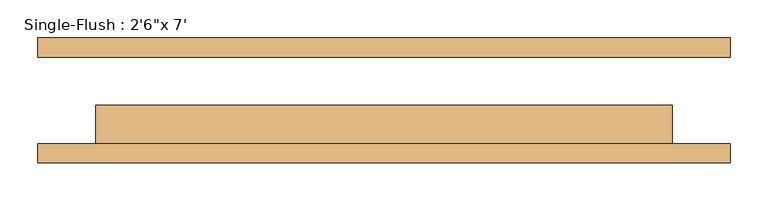
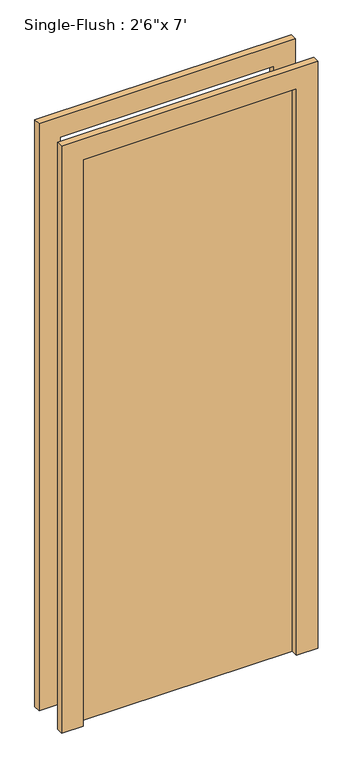
"""IFC4 building model written with IfcOpenShell, lengths in millimetres: door geometry."""

from ifc_helpers import new_model, si_unit, frame, origin, origin_with_axes, place, context, project, spatial, polyline, outline, extrude, source, transform, mapped, element, save


def door_78caadf7(model_context):
    return source(origin(), model_context, "Body", "SweptSolid", [
        extrude(outline(polyline([(2209.8, -457.2), (0.0, -457.2), (0.0, -381.0), (2133.6, -381.0), (2133.6, 381.0), (0.0, 381.0), (0.0, 457.2), (2209.8, 457.2), (2209.8, -457.2)])), frame((0.0, -82.55, 0.0), z_axis=(0.0, 1.0, 0.0), x_axis=(0.0, 0.0, 1.0)), (0.0, 0.0, 1.0), 25.4),
        extrude(outline(polyline([(2209.8, 457.2), (2209.8, -457.2), (0.0, -457.2), (0.0, -381.0), (2133.6, -381.0), (2133.6, 381.0), (0.0, 381.0), (0.0, 457.2), (2209.8, 457.2)])), frame((0.0, 57.15, 0.0), z_axis=(0.0, 1.0, 0.0), x_axis=(0.0, 0.0, 1.0)), (0.0, 0.0, 1.0), 25.4),
        extrude(outline(polyline([(381.0, -6.35), (381.0, -57.15), (-381.0, -57.15), (-381.0, -6.35), (381.0, -6.35)])), origin_with_axes(), (0.0, 0.0, 1.0), 2133.6),
    ])


if __name__ == "__main__":
    model = new_model("IFC4")
    model_context = context("Model", 3, world=origin())
    ifc_project = project(units=[si_unit("LENGTHUNIT", "METRE", prefix="MILLI")], contexts=[model_context])
    site = spatial("IfcSite", under=ifc_project)
    building = spatial("IfcBuilding", under=site)
    placement = place(None, origin())
    door_shape = door_78caadf7(model_context)
    element("IfcDoor", 1, ObjectType="Single-Flush : 2'6\"x 7'", at=placement, inside=building, context=model_context, shape_type="MappedRepresentation", body=[
        mapped(door_shape, transform((0.0, 0.0, 0.0), x_axis=(1.0, 0.0, 0.0), y_axis=(0.0, 1.0, 0.0), z_axis=(0.0, 0.0, 1.0))),
    ])
    save(model, "model.ifc")

# Revit data of these elements
# Type "Single-Flush : 2'6\"x 7'"
#   Type Mark = "8"
#   Construction Type Id = "MDOOR"
#   Assembly Code = "C1020"
#   Analytic Construction = "Metal"
#   Thickness = 0' - 2"
#   Heat Transfer Coefficient (U) = 0.651978 BTU/(h·ft²·°F)
#   Height = 7' - 0"
#   Trim Projection Ext = 0' - 1"
#   Trim Projection Int = 0' - 1"
#   Trim Width = 0' - 3"
#   Width = 2' - 6"
#   Define Thermal Properties by = 1
#   Door Material = Door - Panel
#   Frame Material = Door - Frame
#   Visual Light Transmittance = 0
#   Solar Heat Gain Coefficient = 0
#   Function = (empty or 0)
#   Wall Closure = (empty or 0)
# Element 1 (IfcDoor, "Single-Flush : 2'6\"x 7'")
#   Materials on its faces: "Door - Frame", "Door - Panel"
# Materials
#   "Door - Panel": class "Wood", colour RGB 210 159 95, transparency 0, Cost = 0
#   "Door - Frame": colour RGB 118 70 51, transparency 0, Cost = 0
